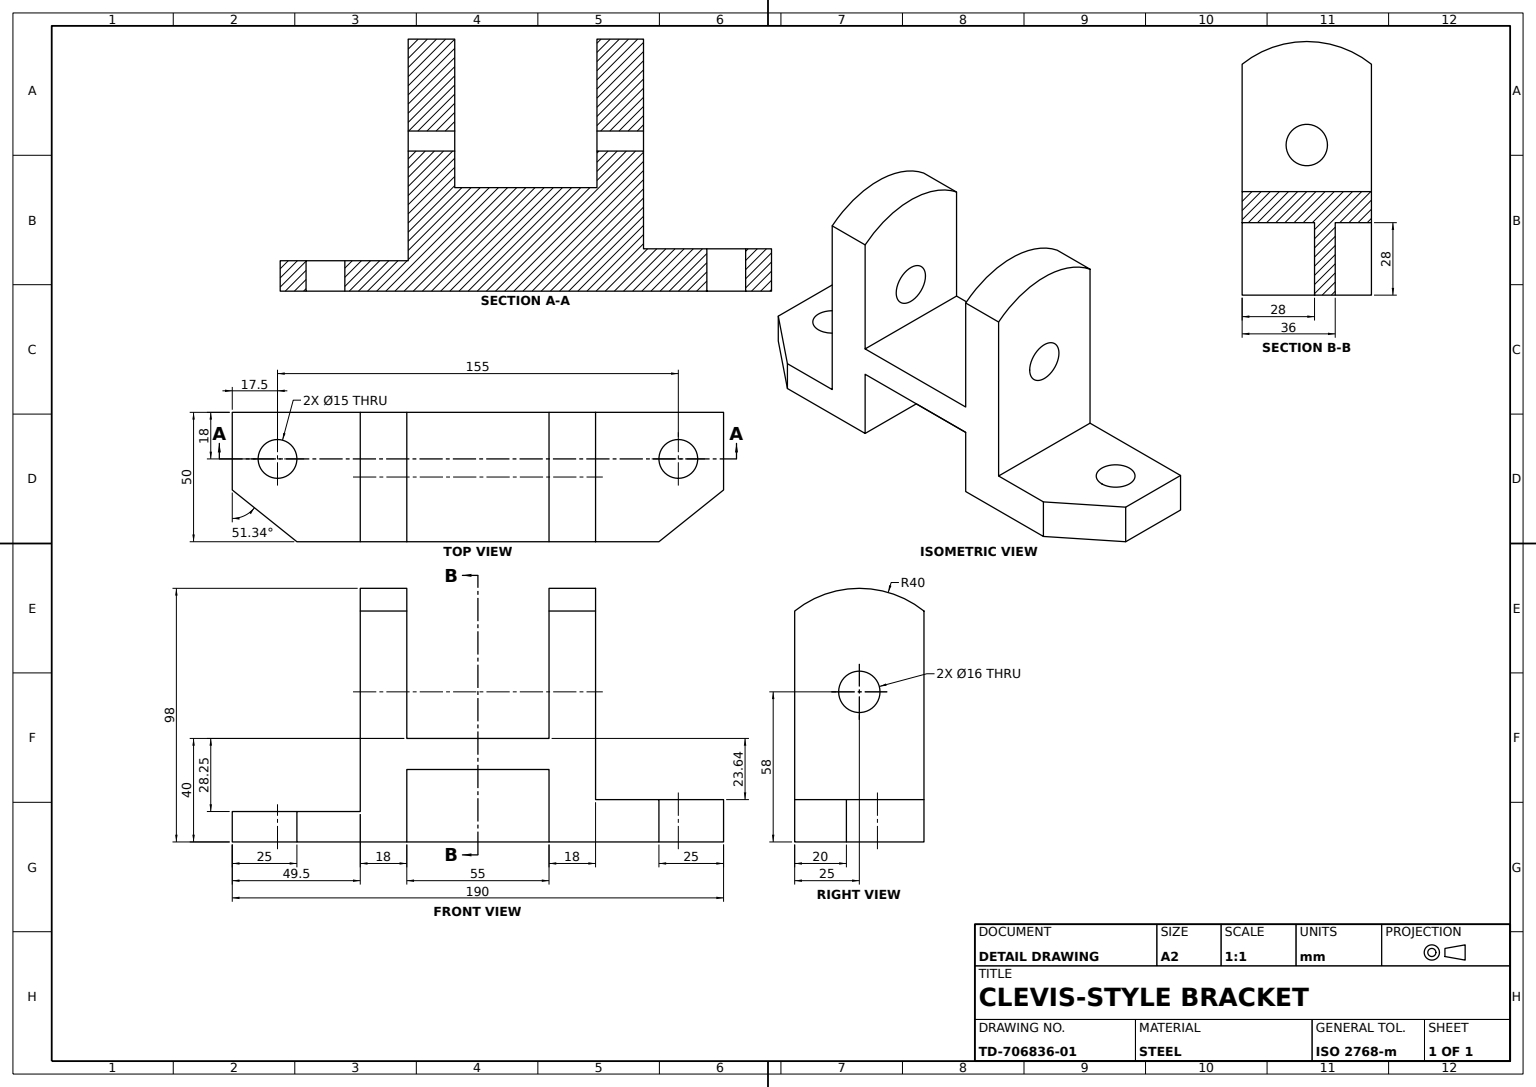
from build123d import *
from OCP.BRepFilletAPI import BRepFilletAPI_MakeChamfer

# Parameters (mm, degrees)
BRACKET_BODY_DEPTH                           = 25
UPRIGHT_ROUNDS_AND_PIN_HOLE_SKETCH_R         = 8
UPRIGHT_ROUNDS_AND_PIN_HOLE_16_DEPTH         = 120
FLANGE_CORNER_CHAMFERS_SIZE                  = 20
FLANGE_CORNER_CHAMFERS_SIZE2                 = 25
MOUNTING_HOLES_AND_RELIEF_SKETCH_R           = 7.5
MOUNTING_HOLES_AND_RELIEF_SKETCH_W           = 55
MOUNTING_HOLES_AND_RELIEF_SKETCH_H           = 28
MOUNTING_HOLES_AND_RELIEF_SKETCH_H_2         = 14
MOUNTING_HOLES_2X_15_AND_CENTRE_RELIEF_DEPTH = 28


with BuildPart() as part:
    # Bracket Side Profile Sketch → Bracket Body (new, symmetric)
    with BuildSketch(Plane.XY):
        Polygon((-95, -28.245219348), (-95, -40), (95, -40), (95, -23.642294713), (45.5, -23.642294713), (45.5, 58), (27.5, 58), (27.5, 0), (-27.5, 0), (-27.5, 58), (-45.5, 58), (-45.5, -28.245219348), align=None)
    extrude(amount=BRACKET_BODY_DEPTH, both=True)

    # Upright Rounds and Pin Hole Sketch → Upright Rounds and Pin Hole Ø16 (cut)
    with BuildSketch(Plane(origin=(45.5, 0, 0), x_dir=(0, 0, -1), z_dir=(1, 0, 0))):
        with BuildLine():
            Line((-25, 58), (-25, 49.224989992))
            ThreePointArc((-25, 49.224989992), (-13.24764886, 55.74254628), (-1.3e-08, 58))
            Line((-1.3e-08, 58), (-25, 58))
        make_face()
        Polygon((-25, 66.800794381), (-25, 58), (-1.3e-08, 58), (25, 58), (25, 66.800794381), align=None)
        with BuildLine():
            Line((25, 58), (-1.3e-08, 58))
            ThreePointArc((-1.3e-08, 58), (13.247648848, 55.742546284), (25, 49.224989992))
            Line((25, 49.224989992), (25, 58))
        make_face()
        with Locations((0, 18)):
            Circle(UPRIGHT_ROUNDS_AND_PIN_HOLE_SKETCH_R)
    extrude(amount=-UPRIGHT_ROUNDS_AND_PIN_HOLE_16_DEPTH, mode=Mode.SUBTRACT)

    # Flange Corner Chamfers: one chamfer whose edges measure the first distance from different faces: ONE call of the kernel's chamfer builder (chamfer() names one face for all edges)
    flange_corner_chamfers_edges_1 = [part.edges().sort_by_distance(p)[0] for p in [
        (95, -31.821147357, 25),
    ]]
    flange_corner_chamfers_side_1 = [part.faces().sort_by_distance(p)[0] for p in [
        (95, -31.821147357, 0),
    ]]
    flange_corner_chamfers_edges_2 = [part.edges().sort_by_distance(p)[0] for p in [
        (-95, -34.122609674, 25),
    ]]
    flange_corner_chamfers_side_2 = [part.faces().sort_by_distance(p)[0] for p in [
        (-95, -34.122609674, 0),
    ]]
    flange_corner_chamfers = BRepFilletAPI_MakeChamfer(part.part.solid().wrapped)
    for e in flange_corner_chamfers_edges_1:
        flange_corner_chamfers.Add(FLANGE_CORNER_CHAMFERS_SIZE, FLANGE_CORNER_CHAMFERS_SIZE2, e.wrapped, flange_corner_chamfers_side_1[0].wrapped)  # the first distance lies on this face
    for e in flange_corner_chamfers_edges_2:
        flange_corner_chamfers.Add(FLANGE_CORNER_CHAMFERS_SIZE, FLANGE_CORNER_CHAMFERS_SIZE2, e.wrapped, flange_corner_chamfers_side_2[0].wrapped)  # the first distance lies on this face
    add(Compound.cast(flange_corner_chamfers.Shape()), mode=Mode.REPLACE)

    # Mounting Holes and Relief Sketch → Mounting Holes 2xØ15 and Centre Relief (cut)
    with BuildSketch(Plane.XZ.offset(40)):
        with Locations(Location((-77.5, -7, 0), (0, 0, 270))):
            Circle(MOUNTING_HOLES_AND_RELIEF_SKETCH_R)
        with Locations(Location((77.5, -7, 0), (0, 0, 270))):
            Circle(MOUNTING_HOLES_AND_RELIEF_SKETCH_R)
        with Locations((0, 11)):
            Rectangle(MOUNTING_HOLES_AND_RELIEF_SKETCH_W, MOUNTING_HOLES_AND_RELIEF_SKETCH_H)
        with Locations((0, -18)):
            Rectangle(MOUNTING_HOLES_AND_RELIEF_SKETCH_W, MOUNTING_HOLES_AND_RELIEF_SKETCH_H_2)
    extrude(amount=-MOUNTING_HOLES_2X_15_AND_CENTRE_RELIEF_DEPTH, mode=Mode.SUBTRACT)


solid = part.part
